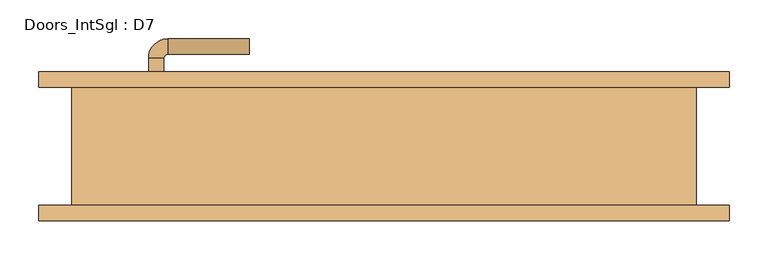
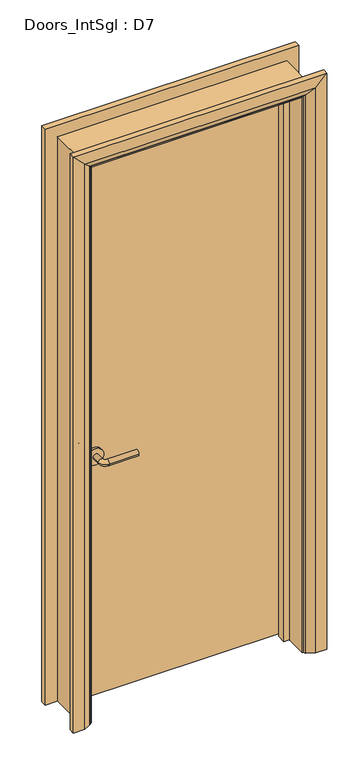
"""IFC4 building model written with IfcOpenShell, lengths in millimetres: door geometry, Doors_IntSgl : D7."""

from ifc_helpers import new_model, si_unit, point, frame, frame_2d, origin, place, context, project, spatial, polyline, circle_curve, ellipse_curve, trimmed, segment, composite_curve, outline, extrude, faceted_brep, source, transform, mapped, element, save
from ifc_brep_helpers import plane_surface, cylinder_surface, revolved_surface, advanced_brep


def doors_intsgl_d7_212e1d6e(model_context):
    return source(origin(), model_context, "Body", "SolidModel", [
        advanced_brep(
        [(-304.48, 30.2, 900.0), (-284.48, 30.2, 900.0), (-284.48, 0.2, 900.0), (-304.48, 0.2, 900.0), (-279.48, -4.8, 900.0), (-279.48, -24.8, 900.0), (-174.48, -24.8, 900.0), (-174.48, -4.8, 900.0)],
        [
            (0, 1, circle_curve(frame((-294.48, 30.2, 900.0), z_axis=(0.0, 1.0, 0.0), x_axis=(1.0, 0.0, 0.0)), 10.0)),
            (1, 0, circle_curve(frame((-294.48, 30.2, 900.0), z_axis=(0.0, 1.0, 0.0), x_axis=(1.0, 0.0, 0.0)), 10.0)),
            (1, 2),
            (2, 3, circle_curve(frame((-294.48, 0.2, 900.0), z_axis=(0.0, 1.0, 0.0), x_axis=(1.0, 0.0, 0.0)), 10.0)),
            (3, 0),
            (3, 2, circle_curve(frame((-294.48, 0.2, 900.0), z_axis=(0.0, 1.0, 0.0), x_axis=(1.0, 0.0, 0.0)), 10.0)),
            (4, 5, circle_curve(frame((-279.48, -14.8, 900.0), z_axis=(-1.0, 0.0, 0.0), x_axis=(0.0, 1.0, 0.0)), 10.0)),
            (5, 3, circle_curve(frame((-279.48, 0.2, 900.0), z_axis=(0.0, 0.0, -1.0), x_axis=(-1.0, 0.0, 0.0)), 25.0)),
            (2, 4, circle_curve(frame((-279.48, 0.2, 900.0), z_axis=(0.0, 0.0, 1.0), x_axis=(-1.0, 0.0, 0.0)), 5.0)),
            (5, 4, circle_curve(frame((-279.48, -14.8, 900.0), z_axis=(-1.0, 0.0, 0.0), x_axis=(0.0, 1.0, 0.0)), 10.0)),
            (6, 7, circle_curve(frame((-174.48, -14.8, 900.0), z_axis=(1.0, 0.0, 0.0), x_axis=(0.0, 1.0, 0.0)), 10.0)),
            (7, 6, circle_curve(frame((-174.48, -14.8, 900.0), z_axis=(1.0, 0.0, 0.0), x_axis=(0.0, 1.0, 0.0)), 10.0)),
            (4, 7),
            (6, 5),
        ],
        [
            plane_surface(frame((-294.48, 30.2, 900.0), z_axis=(0.0, 1.0, 0.0), x_axis=(0.0, 0.0, 1.0))),
            cylinder_surface(frame((-294.48, 30.2, 900.0), z_axis=(0.0, 1.0, 0.0), x_axis=(1.0, 0.0, 0.0)), 10.0),
            revolved_surface(trimmed(ellipse_curve(frame((-294.48, 0.2, 900.0), z_axis=(0.0, -1.0, 0.0), x_axis=(1.0, 0.0, 0.0)), 10.0, 10.0), [point((-304.48, 0.2, 900.0))], [point((-284.48, 0.2, 900.0))], True, "CARTESIAN"), (-279.48, 0.2, 900.0), (0.0, 0.0, -1.0)),
            revolved_surface(trimmed(ellipse_curve(frame((-294.48, 0.2, 900.0), z_axis=(0.0, -1.0, 0.0), x_axis=(1.0, 0.0, 0.0)), 10.0, 10.0), [point((-284.48, 0.2, 900.0))], [point((-304.48, 0.2, 900.0))], True, "CARTESIAN"), (-279.48, 0.2, 900.0), (0.0, 0.0, -1.0)),
            plane_surface(frame((-174.48, -14.8, 900.0), z_axis=(1.0, 0.0, 0.0), x_axis=(0.0, 0.0, 1.0))),
            cylinder_surface(frame((-279.48, -14.8, 900.0), z_axis=(-1.0, 0.0, 0.0), x_axis=(0.0, 1.0, 0.0)), 10.0),
        ],
        [
            (0, [[1, 2]]),
            (1, [[3, 4, 5, -2]]),
            (1, [[-5, 6, -3, -1]]),
            (2, [[7, 8, -4, 9]]),
            (3, [[10, -9, -6, -8]]),
            (4, [[11, 12]]),
            (5, [[13, -11, 14, -7]]),
            (5, [[-14, -12, -13, -10]]),
        ],
    ),
        extrude(outline(composite_curve([segment(trimmed(circle_curve(frame_2d((900.0, -296.98)), 30.0), [point((900.0, -326.98))], [point((900.0, -266.98))], False, "CARTESIAN"), True, "CONTINUOUS"), segment(trimmed(circle_curve(frame_2d((900.0, -296.98)), 30.0), [point((900.0, -266.98))], [point((900.0, -326.98))], False, "CARTESIAN"), True, "CONTINUOUS")], self_intersect=False)), frame((0.0, 30.2, 0.0), z_axis=(0.0, 1.0, 0.0), x_axis=(0.0, 0.0, 1.0)), (0.0, 0.0, 1.0), 8.0),
        advanced_brep(
        [(-304.48, 84.2, 900.0), (-284.48, 84.2, 900.0), (-304.48, 114.2, 900.0), (-284.48, 114.2, 900.0), (-279.48, 119.2, 900.0), (-279.48, 139.2, 900.0), (-174.48, 139.2, 900.0), (-174.48, 119.2, 900.0)],
        [
            (0, 1, circle_curve(frame((-294.48, 84.2, 900.0), z_axis=(0.0, -1.0, 0.0), x_axis=(1.0, 0.0, 0.0)), 10.0)),
            (1, 0, circle_curve(frame((-294.48, 84.2, 900.0), z_axis=(0.0, -1.0, 0.0), x_axis=(1.0, 0.0, 0.0)), 10.0)),
            (0, 2),
            (2, 3, circle_curve(frame((-294.48, 114.2, 900.0), z_axis=(0.0, -1.0, 0.0), x_axis=(1.0, 0.0, 0.0)), 10.0)),
            (3, 1),
            (3, 2, circle_curve(frame((-294.48, 114.2, 900.0), z_axis=(0.0, -1.0, 0.0), x_axis=(1.0, 0.0, 0.0)), 10.0)),
            (4, 3, circle_curve(frame((-279.48, 114.2, 900.0), z_axis=(0.0, 0.0, 1.0), x_axis=(-1.0, 0.0, 0.0)), 5.0)),
            (2, 5, circle_curve(frame((-279.48, 114.2, 900.0), z_axis=(0.0, 0.0, -1.0), x_axis=(-1.0, 0.0, 0.0)), 25.0)),
            (5, 4, circle_curve(frame((-279.48, 129.2, 900.0), z_axis=(-1.0, 0.0, 0.0), x_axis=(0.0, -1.0, 0.0)), 10.0)),
            (4, 5, circle_curve(frame((-279.48, 129.2, 900.0), z_axis=(-1.0, 0.0, 0.0), x_axis=(0.0, -1.0, 0.0)), 10.0)),
            (6, 7, circle_curve(frame((-174.48, 129.2, 900.0), z_axis=(1.0, 0.0, 0.0), x_axis=(0.0, -1.0, 0.0)), 10.0)),
            (7, 6, circle_curve(frame((-174.48, 129.2, 900.0), z_axis=(1.0, 0.0, 0.0), x_axis=(0.0, -1.0, 0.0)), 10.0)),
            (5, 6),
            (7, 4),
        ],
        [
            plane_surface(frame((-294.48, 84.2, 900.0), z_axis=(0.0, -1.0, 0.0), x_axis=(0.0, 0.0, 1.0))),
            cylinder_surface(frame((-294.48, 84.2, 900.0), z_axis=(0.0, -1.0, 0.0), x_axis=(1.0, 0.0, 0.0)), 10.0),
            revolved_surface(trimmed(ellipse_curve(frame((-294.48, 114.2, 900.0), z_axis=(0.0, -1.0, 0.0), x_axis=(1.0, 0.0, 0.0)), 10.0, 10.0), [point((-304.48, 114.2, 900.0))], [point((-284.48, 114.2, 900.0))], True, "CARTESIAN"), (-279.48, 114.2, 900.0), (0.0, 0.0, -1.0)),
            revolved_surface(trimmed(ellipse_curve(frame((-294.48, 114.2, 900.0), z_axis=(0.0, -1.0, 0.0), x_axis=(1.0, 0.0, 0.0)), 10.0, 10.0), [point((-284.48, 114.2, 900.0))], [point((-304.48, 114.2, 900.0))], True, "CARTESIAN"), (-279.48, 114.2, 900.0), (0.0, 0.0, -1.0)),
            plane_surface(frame((-174.48, 129.2, 900.0), z_axis=(1.0, 0.0, 0.0), x_axis=(0.0, 0.0, 1.0))),
            cylinder_surface(frame((-279.48, 129.2, 900.0), z_axis=(-1.0, 0.0, 0.0), x_axis=(0.0, -1.0, 0.0)), 10.0),
        ],
        [
            (0, [[1, 2]]),
            (1, [[-1, 3, 4, 5]]),
            (1, [[-2, -5, 6, -3]]),
            (2, [[7, -4, 8, 9]]),
            (3, [[-8, -6, -7, 10]]),
            (4, [[11, 12]]),
            (5, [[-9, 13, -12, 14]]),
            (5, [[-10, -14, -11, -13]]),
        ],
    ),
        extrude(outline(composite_curve([segment(trimmed(circle_curve(frame_2d((900.0, -296.98)), 30.0), [point((900.0, -326.98))], [point((900.0, -266.98))], False, "CARTESIAN"), True, "CONTINUOUS"), segment(trimmed(circle_curve(frame_2d((900.0, -296.98)), 30.0), [point((900.0, -266.98))], [point((900.0, -326.98))], False, "CARTESIAN"), True, "CONTINUOUS")], self_intersect=False)), frame((0.0, 76.2, 0.0), z_axis=(0.0, 1.0, 0.0), x_axis=(0.0, 0.0, 1.0)), (0.0, 0.0, 1.0), 8.0),
        extrude(outline(polyline([(369.48, 38.2), (-369.48, 38.2), (-369.48, 76.2), (369.48, 76.2), (369.48, 38.2)])), frame((0.0, 0.0, 8.0), z_axis=(0.0, 0.0, 1.0), x_axis=(1.0, 0.0, 0.0)), (0.0, 0.0, 1.0), 2060.0),
        advanced_brep(
        [(446.48, 96.2, 0.0), (446.48, 76.2, 0.0), (376.48, 76.2, 0.0), (380.48, 82.2, 0.0), (406.48, 96.2, 0.0), (446.48, 96.2, 2145.0), (446.48, 76.2, 2145.0), (-446.48, 76.2, 2145.0), (-446.48, 76.2, 0.0), (-376.48, 76.2, 0.0), (-376.48, 76.2, 2075.0), (376.48, 76.2, 2075.0), (380.48, 82.2, 2079.0), (406.48, 96.2, 2105.0), (-406.48, 96.2, 2105.0), (-406.48, 96.2, 0.0), (-446.48, 96.2, 0.0), (-446.48, 96.2, 2145.0), (-380.48, 82.2, 0.0), (-380.48, 82.2, 2079.0)],
        [
            (0, 1),
            (1, 2),
            (2, 3, circle_curve(frame((384.48, 75.2, 0.0), z_axis=(0.0, 0.0, -1.0), x_axis=(1.0, 0.0, 0.0)), 8.0622577)),
            (3, 4),
            (4, 0),
            (0, 5),
            (5, 6),
            (6, 1),
            (6, 7),
            (7, 8),
            (8, 9),
            (9, 10),
            (10, 11),
            (11, 2),
            (11, 12, ellipse_curve(frame((384.48, 75.2, 2083.0), z_axis=(0.7071067811865475, 0.0, -0.7071067811865475), x_axis=(-0.7071067811865474, 0.0, -0.7071067811865476)), 11.4017543, 8.0622577)),
            (12, 3),
            (12, 13),
            (13, 4),
            (13, 14),
            (14, 15),
            (15, 16),
            (16, 17),
            (17, 5),
            (7, 17),
            (16, 8),
            (15, 18),
            (18, 9, circle_curve(frame((-384.48, 75.2, 0.0), z_axis=(0.0, 0.0, -1.0), x_axis=(-1.0, 0.0, 0.0)), 8.0622577)),
            (19, 10, ellipse_curve(frame((-384.48, 75.2, 2083.0), z_axis=(-0.7071067811865475, 0.0, -0.7071067811865475), x_axis=(-0.7071067811865474, 0.0, 0.7071067811865476)), 11.4017543, 8.0622577)),
            (18, 19),
            (14, 19),
            (19, 12),
        ],
        [
            plane_surface(frame((376.48, 76.2, 0.0), z_axis=(0.0, 0.0, -1.0), x_axis=(0.0, -1.0, 0.0))),
            plane_surface(frame((446.48, 96.2, 0.0), z_axis=(1.0, 0.0, 0.0), x_axis=(0.0, 0.0, 1.0))),
            plane_surface(frame((446.48, 76.2, 0.0), z_axis=(0.0, -1.0, 0.0), x_axis=(0.0, 0.0, 1.0))),
            cylinder_surface(frame((384.48, 75.2, 0.0), z_axis=(0.0, 0.0, -1.0), x_axis=(1.0, 0.0, 0.0)), 8.0622577),
            plane_surface(frame((380.48, 82.2, 0.0), z_axis=(-0.4740998230350126, 0.880471099922178, 0.0), x_axis=(0.0, 0.0, 1.0))),
            plane_surface(frame((406.48, 96.2, 0.0), z_axis=(0.0, 1.0, 0.0), x_axis=(0.0, 0.0, 1.0))),
            plane_surface(frame((-446.48, 96.2, 2145.0), z_axis=(-1.0, 0.0, 0.0), x_axis=(0.0, 0.0, -1.0))),
            plane_surface(frame((-376.48, 76.2, 0.0), z_axis=(0.0, 0.0, -1.0), x_axis=(0.0, -1.0, 0.0))),
            cylinder_surface(frame((-384.48, 75.2, 2075.0), z_axis=(0.0, 0.0, 1.0), x_axis=(-1.0, 0.0, 0.0)), 8.0622577),
            plane_surface(frame((-380.48, 82.2, 2079.0), z_axis=(0.47409982303501824, 0.8804710999221749, 0.0), x_axis=(0.0, 0.0, -1.0))),
            plane_surface(frame((446.48, 96.2, 2145.0), z_axis=(0.0, 0.0, 1.0), x_axis=(-1.0, 0.0, 0.0))),
            cylinder_surface(frame((376.48, 75.2, 2083.0), z_axis=(1.0, 0.0, 0.0), x_axis=(0.0, 0.0, 1.0)), 8.0622577),
            plane_surface(frame((380.48, 82.2, 2079.0), z_axis=(0.0, 0.8804710999221764, -0.4740998230350154), x_axis=(-1.0, 0.0, 0.0))),
        ],
        [
            (0, [[1, 2, 3, 4, 5]]),
            (1, [[-1, 6, 7, 8]]),
            (2, [[-2, -8, 9, 10, 11, 12, 13, 14]]),
            (3, [[-3, -14, 15, 16]]),
            (4, [[-4, -16, 17, 18]]),
            (5, [[-5, -18, 19, 20, 21, 22, 23, -6]]),
            (6, [[24, -22, 25, -10]]),
            (7, [[-21, 26, 27, -11, -25]]),
            (8, [[28, -12, -27, 29]]),
            (9, [[30, -29, -26, -20]]),
            (10, [[-7, -23, -24, -9]]),
            (11, [[-15, -13, -28, 31]]),
            (12, [[-17, -31, -30, -19]]),
        ],
    ),
        extrude(outline(polyline([(0.0, -371.48), (0.0, -352.48), (2051.0, -352.48), (2051.0, 352.48), (0.0, 352.48), (0.0, 371.48), (2070.0, 371.48), (2070.0, -371.48), (0.0, -371.48)])), frame((0.0, 4.2, 0.0), z_axis=(0.0, 1.0, 0.0), x_axis=(0.0, 0.0, 1.0)), (0.0, 0.0, 1.0), 32.0),
        advanced_brep(
        [(-446.48, -96.2, 0.0), (-446.48, -76.2, 0.0), (-376.48, -76.2, 0.0), (-380.48, -82.2, 0.0), (-406.48, -96.2, 0.0), (-446.48, -96.2, 2145.0), (-446.48, -76.2, 2145.0), (-376.48, -76.2, 2075.0), (-380.48, -82.2, 2079.0), (-406.48, -96.2, 2105.0), (446.48, -96.2, 0.0), (406.48, -96.2, 0.0), (380.48, -82.2, 0.0), (376.48, -76.2, 0.0), (446.48, -76.2, 0.0), (446.48, -96.2, 2145.0), (406.48, -96.2, 2105.0), (380.48, -82.2, 2079.0), (376.48, -76.2, 2075.0), (446.48, -76.2, 2145.0)],
        [
            (0, 1),
            (1, 2),
            (2, 3, circle_curve(frame((-384.48, -75.2, 0.0), z_axis=(0.0, 0.0, -1.0), x_axis=(-1.0, 0.0, 0.0)), 8.0622577)),
            (3, 4),
            (4, 0),
            (0, 5),
            (5, 6),
            (6, 1),
            (6, 7),
            (7, 2),
            (7, 8, ellipse_curve(frame((-384.48, -75.2, 2083.0), z_axis=(-0.7071067811865475, 0.0, -0.7071067811865475), x_axis=(0.7071067811865474, 0.0, -0.7071067811865476)), 11.4017543, 8.0622577)),
            (8, 3),
            (8, 9),
            (9, 4),
            (9, 5),
            (10, 11),
            (11, 12),
            (12, 13, circle_curve(frame((384.48, -75.2, 0.0), z_axis=(0.0, 0.0, -1.0), x_axis=(1.0, 0.0, 0.0)), 8.0622577)),
            (13, 14),
            (14, 10),
            (15, 16),
            (16, 11),
            (10, 15),
            (16, 17),
            (17, 12),
            (17, 18, ellipse_curve(frame((384.48, -75.2, 2083.0), z_axis=(0.7071067811865475, 0.0, -0.7071067811865475), x_axis=(0.7071067811865474, 0.0, 0.7071067811865476)), 11.4017543, 8.0622577)),
            (18, 13),
            (18, 19),
            (19, 14),
            (19, 15),
            (5, 15),
            (19, 6),
            (18, 7),
            (17, 8),
            (16, 9),
        ],
        [
            plane_surface(frame((-376.48, -149.0010989, 0.0), z_axis=(0.0, 0.0, -1.0), x_axis=(1.0, 0.0, 0.0))),
            plane_surface(frame((-446.48, -96.2, 0.0), z_axis=(-1.0, 0.0, 0.0), x_axis=(0.0, 0.0, 1.0))),
            plane_surface(frame((-446.48, -76.2, 0.0), z_axis=(0.0, 1.0, 0.0), x_axis=(0.0, 0.0, 1.0))),
            cylinder_surface(frame((-384.48, -75.2, 0.0), z_axis=(0.0, 0.0, -1.0), x_axis=(-1.0, 0.0, 0.0)), 8.0622577),
            plane_surface(frame((-380.48, -82.2, 0.0), z_axis=(0.4740998230350183, -0.8804710999221749, 0.0), x_axis=(0.0, 0.0, 1.0))),
            plane_surface(frame((-406.48, -96.2, 0.0), z_axis=(0.0, -1.0, 0.0), x_axis=(0.0, 0.0, 1.0))),
            plane_surface(frame((376.48, -149.0010989, 0.0), z_axis=(0.0, 0.0, -1.0), x_axis=(-1.0, 0.0, 0.0))),
            plane_surface(frame((406.48, -96.2, 2105.0), z_axis=(0.0, -1.0, 0.0), x_axis=(0.0, 0.0, -1.0))),
            plane_surface(frame((380.48, -82.2, 2079.0), z_axis=(-0.4740998230350183, -0.8804710999221749, 0.0), x_axis=(0.0, 0.0, -1.0))),
            cylinder_surface(frame((384.48, -75.2, 2075.0), z_axis=(0.0, 0.0, 1.0), x_axis=(1.0, 0.0, 0.0)), 8.0622577),
            plane_surface(frame((446.48, -76.2, 2145.0), z_axis=(0.0, 1.0, 0.0), x_axis=(0.0, 0.0, -1.0))),
            plane_surface(frame((446.48, -96.2, 2145.0), z_axis=(1.0, 0.0, 0.0), x_axis=(0.0, 0.0, -1.0))),
            plane_surface(frame((-446.48, -96.2, 2145.0), z_axis=(0.0, 0.0, 1.0), x_axis=(1.0, 0.0, 0.0))),
            plane_surface(frame((-446.48, -76.2, 2145.0), z_axis=(0.0, 1.0, 0.0), x_axis=(1.0, 0.0, 0.0))),
            cylinder_surface(frame((-376.48, -75.2, 2083.0), z_axis=(-1.0, 0.0, 0.0), x_axis=(0.0, 0.0, 1.0)), 8.0622577),
            plane_surface(frame((-380.48, -82.2, 2079.0), z_axis=(0.0, -0.8804710999221749, -0.4740998230350183), x_axis=(1.0, 0.0, 0.0))),
            plane_surface(frame((-406.48, -96.2, 2105.0), z_axis=(0.0, -1.0, 0.0), x_axis=(1.0, 0.0, 0.0))),
        ],
        [
            (0, [[1, 2, 3, 4, 5]]),
            (1, [[-1, 6, 7, 8]]),
            (2, [[-2, -8, 9, 10]]),
            (3, [[-3, -10, 11, 12]]),
            (4, [[-4, -12, 13, 14]]),
            (5, [[-5, -14, 15, -6]]),
            (6, [[16, 17, 18, 19, 20]]),
            (7, [[21, 22, -16, 23]]),
            (8, [[24, 25, -17, -22]]),
            (9, [[26, 27, -18, -25]]),
            (10, [[28, 29, -19, -27]]),
            (11, [[30, -23, -20, -29]]),
            (12, [[-7, 31, -30, 32]]),
            (13, [[-9, -32, -28, 33]]),
            (14, [[-11, -33, -26, 34]]),
            (15, [[-13, -34, -24, 35]]),
            (16, [[-15, -35, -21, -31]]),
        ],
    ),
        faceted_brep([(-371.48, 76.2, 0.0), (-371.48, -76.2, 0.0), (-403.48, -76.2, 0.0), (-403.48, 76.2, 0.0), (-371.48, 76.2, 2070.0), (-371.48, -76.2, 2070.0), (-403.48, -76.2, 2102.0), (-403.48, 76.2, 2102.0), (371.48, 76.2, 0.0), (403.48, 76.2, 0.0), (403.48, -76.2, 0.0), (371.48, -76.2, 0.0), (371.48, 76.2, 2070.0), (403.48, 76.2, 2102.0), (403.48, -76.2, 2102.0), (371.48, -76.2, 2070.0)], [[[0, 1, 2, 3]], [[1, 0, 4, 5]], [[2, 1, 5, 6]], [[3, 2, 6, 7]], [[0, 3, 7, 4]], [[8, 9, 10, 11]], [[12, 13, 9, 8]], [[13, 14, 10, 9]], [[14, 15, 11, 10]], [[15, 12, 8, 11]], [[5, 4, 12, 15]], [[6, 5, 15, 14]], [[7, 6, 14, 13]], [[4, 7, 13, 12]]]),
    ])


if __name__ == "__main__":
    model = new_model("IFC4")
    model_context = context("Model", 3, world=origin())
    ifc_project = project(units=[si_unit("LENGTHUNIT", "METRE", prefix="MILLI")], contexts=[model_context])
    site = spatial("IfcSite", under=ifc_project)
    building = spatial("IfcBuilding", under=site)
    placement = place(None, origin())
    doors_intsgl_d7_shape = doors_intsgl_d7_212e1d6e(model_context)
    element("IfcDoor", 1, ObjectType="Doors_IntSgl : D7", at=placement, inside=building, context=model_context, shape_type="MappedRepresentation", body=[
        mapped(doors_intsgl_d7_shape, transform((0.0, 0.0, 0.0), x_axis=(1.0, 0.0, 0.0), y_axis=(0.0, 1.0, 0.0), z_axis=(0.0, 0.0, 1.0))),
    ])
    save(model, "model.ifc")

# Revit data of these elements
# Type "Doors_IntSgl : D7"
#   Type Mark = "46"
#   Type Comments = "Internal Single"
#   Operation = "SingleSwingRight"
#   Manufacturer = "Revit"
#   Keynote = "L20"
#   Description = "Internal Single Door"
#   Analytic Construction = "Metal"
#   UnderCut = 0.026247 ft
#   Tolerance = 0.006562 ft
#   Thickness = 0.124672 ft
#   Thermal Resistance (R) = 0.270117 (m²·K)/W
#   Structural Tolerance = 0.026247 ft
#   StopDepth = 0.104987 ft
#   Stop Thickness = 0.062336 ft
#   Rough Width = 2.7 ft
#   Rough Height = 6.922572 ft
#   Height to Top Lock Rail = 3.28084 ft
#   Heat Transfer Coefficient (U) = 3.7021 W/(m²·K)
#   Handle Z Distance = 2.952756 ft
#   Handle X Distance = 0.246063 ft
#   Frame Thickness = 0.104987 ft
#   Door Panel Width = 2.424409 ft
#   Door Panel Thickness = 0.124672 ft
#   Door Panel Offset = 0.0 ft
#   Height = 6.922572 ft
#   Width = 2.7 ft
#   Door Panel Height = 6.75853 ft
#   Architrave Setback = 0.016404 ft
#   Vis - Ironmongery = yes
#   Material Ironmongery = Door - Handle
#   Material Frame = Door - Frame/Mullion (1)
#   Material Door = Door - Panel
#   Material Architrave = Door - Architrave
#   Visual Light Transmittance = 0
#   Solar Heat Gain Coefficient = 0
#   Function = (empty or 0)
#   Wall Closure = (empty or 0)
# Element 1 (IfcDoor, "Doors_IntSgl : D7")
#   Materials on its faces: "Door - Architrave", "Door - Handle", "Door - Frame/Mullion (1)", "Door - Panel"
# Materials
#   "Door - Handle": colour RGB 0 0 0, transparency 0, Keynote = "P21", Cost = 0
#   "Door - Frame/Mullion (1)": class "Wood", colour RGB 212 179 113, transparency 0, Keynote = "L20", Cost = 0
#   "Door - Panel": class "Wood", colour RGB 210 159 95, transparency 0, Keynote = "L20", Cost = 0
#   "Door - Architrave": class "Wood", colour RGB 154 90 5, transparency 0, Keynote = "P20", Cost = 0
